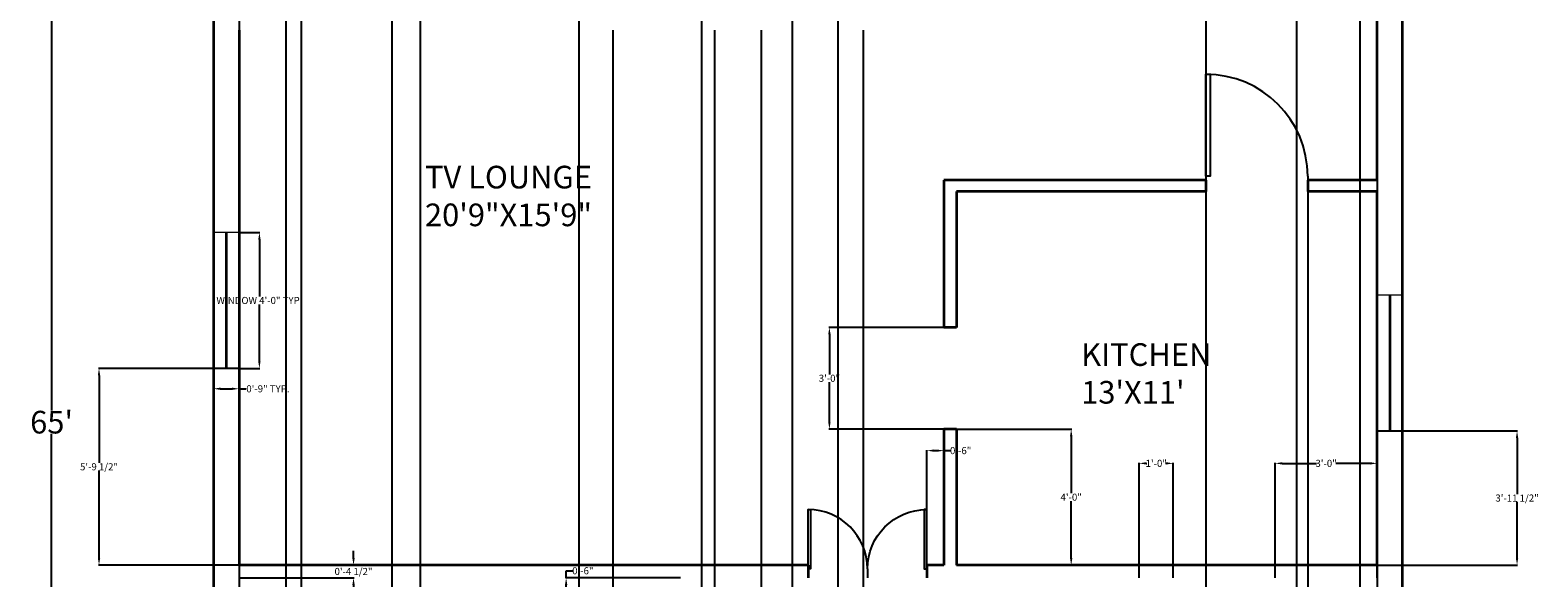
# Model space of a CAD drawing. Units: inches. Extents: x 1737 to 2270, y 2551 to 3419.
# Tile 3 of 4: x 1737 to 2270, y 2930 to 3124. Entities that reach past the tile are written whole.
import ezdxf

# ---------------------------------------------------------------- set-up
doc = ezdxf.new("R2010")
doc.units = ezdxf.units.IN
doc.header["$MEASUREMENT"] = 0
doc.layers.get('0').update_dxf_attribs({"color": 60})
for name, color, linetype, lineweight in [('A-ANNO-DIMS', 2, 'Continuous', 18), ('A-AREA-IDEN', 231, 'Continuous', 18), ('DOOR', 20, 'Continuous', 25), ('WALL', 60, 'Continuous', 35), ('WINDOW', 30, 'Continuous', 18)]:
    doc.layers.add(name, color=color, linetype=linetype, lineweight=lineweight)
doc.styles.get("Standard").update_dxf_attribs({"font": 'arial.ttf'})
doc.dimstyles.get("Standard").update_dxf_attribs({"dimtxt": 2.5, "dimasz": 2.5, "dimexe": 0.18, "dimexo": 0.0625, "dimgap": 0.09, "dimtad": 0, "dimtih": 1, "dimtoh": 1, "dimzin": 0, "dimdsep": 46, "dimlunit": 3, "dimtxsty": 'Standard', "dimcen": 0.09, "dimadec": 0, "dimazin": 0, "dimtfac": 1, "dimtofl": 0, "dimtmove": 0, "dimatfit": 3, "dimfxl": 1, "dimtolj": 1, "dimtzin": 0, "dimarcsym": 0})

# ---------------------------------------------------------------- blocks, each defined once
blk = doc.blocks.new('*U2')
for p, q in [((0, 0), (0, -6)), ((40, 0), (40, -6))]:
    blk.add_line(p, q)
blk.add_lwpolyline([(0, 0), (0, 40), (1.75, 40), (1.75, 0)], close=True)
blk.add_arc((0, 0), 40, 0, 90)
blk = doc.blocks.new('*D5')
at = {"layer": 'A-ANNO-DIMS', "color": 0, "lineweight": -2, "transparency": 16777216}
for p, q in [((1802.15, 3375.16), (1744.83, 3375.16)), ((1745.01, 3372.66), (1745.01, 2989.33)), ((1745.01, 2597.66), (1745.01, 2980.98)), ((1802.15, 2595.16), (1744.83, 2595.16))]:
    blk.add_line(p, q, dxfattribs=at)
at = {"layer": 'A-ANNO-DIMS', "color": 0, "transparency": 16777216}
for points in [[(1744.59, 3372.66), (1745.42, 3372.66), (1745.01, 3375.16)], [(1744.59, 2597.66), (1745.42, 2597.66), (1745.01, 2595.16)]]:
    blk.add_solid(points, dxfattribs=at)
at = {"layer": 'Defpoints', "color": 0, "transparency": 16777216}
for p in [(1802.21, 3375.16), (1745.01, 2595.16), (1802.21, 2595.16)]:
    blk.add_point(p, dxfattribs=at)
at = {"layer": 'A-ANNO-DIMS', "color": 0, "transparency": 16777216, "insert": (1745.01, 2985.16), "char_height": 8, "attachment_point": 5}
blk.add_mtext("\\A1;65'", dxfattribs=at)
blk = doc.blocks.new('WIN-48IN')
for p, q in [((4.25, 48), (4.25, 0)), ((4.75, 48), (4.75, 0))]:
    blk.add_line(p, q)
blk.add_lwpolyline([(0, 48), (0, 0), (9, 0), (9, 48)], close=True)
blk = doc.blocks.new('*D9')
at = {"layer": 'A-ANNO-DIMS', "color": 0, "lineweight": -2, "transparency": 16777216}
for p, q in [((1811.27, 3052.16), (1818.59, 3052.16)), ((1818.41, 3049.66), (1818.41, 3029.55)), ((1818.41, 3006.66), (1818.41, 3026.78)), ((1811.27, 3004.16), (1818.59, 3004.16))]:
    blk.add_line(p, q, dxfattribs=at)
at = {"layer": 'A-ANNO-DIMS', "color": 0, "transparency": 16777216}
for points in [[(1817.99, 3049.66), (1818.83, 3049.66), (1818.41, 3052.16)], [(1817.99, 3006.66), (1818.83, 3006.66), (1818.41, 3004.16)]]:
    blk.add_solid(points, dxfattribs=at)
at = {"layer": 'Defpoints', "color": 0, "transparency": 16777216}
for p in [(1811.21, 3052.16), (1818.41, 3052.16), (1811.21, 3004.16)]:
    blk.add_point(p, dxfattribs=at)
at = {"layer": 'A-ANNO-DIMS', "color": 0, "transparency": 16777216, "insert": (1818.41, 3028.16), "char_height": 2.5, "attachment_point": 5}
blk.add_mtext('\\A1;WINDOW 4\'-0" TYP.', dxfattribs=at)
blk = doc.blocks.new('*D10')
at = {"layer": 'A-ANNO-DIMS', "color": 0, "lineweight": -2, "transparency": 16777216}
for p, q in [((1802.21, 3004.1), (1802.21, 2996.78)), ((1811.21, 3004.1), (1811.21, 2996.78)), ((1804.71, 2996.96), (1808.71, 2996.96)), ((1811.21, 2996.96), (1813.71, 2996.96))]:
    blk.add_line(p, q, dxfattribs=at)
at = {"layer": 'A-ANNO-DIMS', "color": 0, "transparency": 16777216}
for points in [[(1804.71, 2997.38), (1804.71, 2996.55), (1802.21, 2996.96)], [(1808.71, 2997.38), (1808.71, 2996.55), (1811.21, 2996.96)]]:
    blk.add_solid(points, dxfattribs=at)
at = {"layer": 'Defpoints', "color": 0, "transparency": 16777216}
for p in [(1802.21, 3004.16), (1811.21, 3004.16), (1811.21, 2996.96)]:
    blk.add_point(p, dxfattribs=at)
at = {"layer": 'A-ANNO-DIMS', "color": 0, "transparency": 16777216, "insert": (1821.42, 2996.96), "char_height": 2.5, "attachment_point": 5}
blk.add_mtext('\\A1;0\'-9" TYP.', dxfattribs=at)
blk = doc.blocks.new('*D14')
at = {"layer": 'A-ANNO-DIMS', "color": 0, "lineweight": -2, "transparency": 16777216}
for p, q in [((1811.15, 3004.16), (1761.58, 3004.16)), ((1761.76, 3001.66), (1761.76, 2970.79)), ((1761.76, 2937.16), (1761.76, 2968.03)), ((1811.15, 2934.66), (1761.58, 2934.66))]:
    blk.add_line(p, q, dxfattribs=at)
at = {"layer": 'A-ANNO-DIMS', "color": 0, "transparency": 16777216}
for points in [[(1761.34, 3001.66), (1762.18, 3001.66), (1761.76, 3004.16)], [(1761.34, 2937.16), (1762.18, 2937.16), (1761.76, 2934.66)]]:
    blk.add_solid(points, dxfattribs=at)
at = {"layer": 'Defpoints', "color": 0, "transparency": 16777216}
for p in [(1761.76, 3004.16), (1811.21, 3004.16), (1811.21, 2934.66)]:
    blk.add_point(p, dxfattribs=at)
at = {"layer": 'A-ANNO-DIMS', "color": 0, "transparency": 16777216, "insert": (1761.76, 2969.41), "char_height": 2.5, "attachment_point": 5}
blk.add_mtext('\\A1;5\'-9 1/2"', dxfattribs=at)
blk = doc.blocks.new('*D16')
at = {"layer": 'A-ANNO-DIMS', "color": 0, "lineweight": -2, "transparency": 16777216}
for p, q in [((2213.27, 2982.05), (2262.84, 2982.05)), ((2262.66, 2979.55), (2262.66, 2959.74)), ((2262.66, 2937.16), (2262.66, 2956.97)), ((2213.27, 2934.66), (2262.84, 2934.66))]:
    blk.add_line(p, q, dxfattribs=at)
at = {"layer": 'A-ANNO-DIMS', "color": 0, "transparency": 16777216}
for points in [[(2262.24, 2979.55), (2263.08, 2979.55), (2262.66, 2982.05)], [(2262.24, 2937.16), (2263.08, 2937.16), (2262.66, 2934.66)]]:
    blk.add_solid(points, dxfattribs=at)
at = {"layer": 'Defpoints', "color": 0, "transparency": 16777216}
for p in [(2213.21, 2982.05), (2262.66, 2982.05), (2213.21, 2934.66)]:
    blk.add_point(p, dxfattribs=at)
at = {"layer": 'A-ANNO-DIMS', "color": 0, "transparency": 16777216, "insert": (2262.66, 2958.35), "char_height": 2.5, "attachment_point": 5}
blk.add_mtext('\\A1;3\'-11 1/2"', dxfattribs=at)
blk = doc.blocks.new('*D18')
at = {"layer": 'A-ANNO-DIMS', "color": 0, "lineweight": -2, "transparency": 16777216}
for p, q in [((1811.21, 3366.1), (1811.21, 2554.53)), ((1827.73, 3366.1), (1827.73, 2554.53)), ((1808.71, 2554.71), (1806.21, 2554.71)), ((1830.23, 2554.71), (1832.73, 2554.71))]:
    blk.add_line(p, q, dxfattribs=at)
at = {"layer": 'A-ANNO-DIMS', "color": 0, "transparency": 16777216}
for points in [[(1808.71, 2555.12), (1808.71, 2554.29), (1811.21, 2554.71)], [(1830.23, 2555.12), (1830.23, 2554.29), (1827.73, 2554.71)]]:
    blk.add_solid(points, dxfattribs=at)
at = {"layer": 'Defpoints', "color": 0, "transparency": 16777216}
for p in [(1811.21, 3366.16), (1827.73, 3366.16), (1827.73, 2554.71)]:
    blk.add_point(p, dxfattribs=at)
at = {"layer": 'A-ANNO-DIMS', "color": 0, "transparency": 16777216, "insert": (1819.47, 2554.71), "char_height": 2.5, "attachment_point": 5}
blk.add_mtext('\\A1;1\'-4 1/2"', dxfattribs=at)
blk = doc.blocks.new('*D20')
at = {"layer": 'A-ANNO-DIMS', "color": 0, "lineweight": -2, "transparency": 16777216}
for p, q in [((2022.87, 2595.22), (2022.87, 3415.79)), ((2025.37, 3415.61), (2107.86, 3415.61)), ((2204.71, 3415.61), (2122.22, 3415.61)), ((2207.21, 2595.22), (2207.21, 3415.79))]:
    blk.add_line(p, q, dxfattribs=at)
at = {"layer": 'A-ANNO-DIMS', "color": 0, "transparency": 16777216}
for points in [[(2025.37, 3416.02), (2025.37, 3415.19), (2022.87, 3415.61)], [(2204.71, 3416.02), (2204.71, 3415.19), (2207.21, 3415.61)]]:
    blk.add_solid(points, dxfattribs=at)
at = {"layer": 'Defpoints', "color": 0, "transparency": 16777216}
for p in [(2207.21, 3415.61), (2022.87, 2595.16), (2207.21, 2595.16)]:
    blk.add_point(p, dxfattribs=at)
at = {"layer": 'A-ANNO-DIMS', "color": 0, "transparency": 16777216, "insert": (2115.04, 3415.61), "char_height": 2.5, "attachment_point": 5}
blk.add_mtext('\\A1;15\'-4 1/2"', dxfattribs=at)
blk = doc.blocks.new('*D23')
at = {"layer": 'A-ANNO-DIMS', "color": 0, "lineweight": -2, "transparency": 16777216}
for p, q in [((1943.21, 3123.6), (1943.21, 2554.53)), ((1979.21, 3123.6), (1979.21, 2554.53)), ((1945.71, 2554.71), (1957.8, 2554.71)), ((1976.71, 2554.71), (1964.62, 2554.71))]:
    blk.add_line(p, q, dxfattribs=at)
at = {"layer": 'A-ANNO-DIMS', "color": 0, "transparency": 16777216}
for points in [[(1945.71, 2555.12), (1945.71, 2554.29), (1943.21, 2554.71)], [(1976.71, 2555.12), (1976.71, 2554.29), (1979.21, 2554.71)]]:
    blk.add_solid(points, dxfattribs=at)
at = {"layer": 'Defpoints', "color": 0, "transparency": 16777216}
for p in [(1943.21, 3123.66), (1979.21, 3123.66), (1979.21, 2554.71)]:
    blk.add_point(p, dxfattribs=at)
at = {"layer": 'A-ANNO-DIMS', "color": 0, "transparency": 16777216, "insert": (1961.21, 2554.71), "char_height": 2.5, "attachment_point": 5}
blk.add_mtext('\\A1;3\'-0"', dxfattribs=at)
blk = doc.blocks.new('*D24')
at = {"layer": 'A-ANNO-DIMS', "color": 0, "lineweight": -2, "transparency": 16777216}
for p, q in [((1833.21, 3284.1), (1833.21, 2554.53)), ((1865.21, 3284.1), (1865.21, 2554.53)), ((1835.71, 2554.71), (1845.77, 2554.71)), ((1862.71, 2554.71), (1852.64, 2554.71))]:
    blk.add_line(p, q, dxfattribs=at)
at = {"layer": 'A-ANNO-DIMS', "color": 0, "transparency": 16777216}
for points in [[(1835.71, 2555.12), (1835.71, 2554.29), (1833.21, 2554.71)], [(1862.71, 2555.12), (1862.71, 2554.29), (1865.21, 2554.71)]]:
    blk.add_solid(points, dxfattribs=at)
at = {"layer": 'Defpoints', "color": 0, "transparency": 16777216}
for p in [(1833.21, 3284.16), (1865.21, 3284.16), (1865.21, 2554.71)]:
    blk.add_point(p, dxfattribs=at)
at = {"layer": 'A-ANNO-DIMS', "color": 0, "transparency": 16777216, "insert": (1849.21, 2554.71), "char_height": 2.5, "attachment_point": 5}
blk.add_mtext('\\A1;2\'-8"', dxfattribs=at)
blk = doc.blocks.new('*D26')
at = {"layer": 'A-ANNO-DIMS', "color": 0, "lineweight": -2, "transparency": 16777216}
for p, q in [((2060.15, 3018.66), (2019.58, 3018.66)), ((2019.76, 3016.16), (2019.76, 3002.03)), ((2019.76, 2985.16), (2019.76, 2999.29)), ((2060.15, 2982.66), (2019.58, 2982.66))]:
    blk.add_line(p, q, dxfattribs=at)
at = {"layer": 'A-ANNO-DIMS', "color": 0, "transparency": 16777216}
for points in [[(2019.34, 3016.16), (2020.18, 3016.16), (2019.76, 3018.66)], [(2019.34, 2985.16), (2020.18, 2985.16), (2019.76, 2982.66)]]:
    blk.add_solid(points, dxfattribs=at)
at = {"layer": 'Defpoints', "color": 0, "transparency": 16777216}
for p in [(2019.76, 3018.66), (2060.21, 3018.66), (2060.21, 2982.66)]:
    blk.add_point(p, dxfattribs=at)
at = {"layer": 'A-ANNO-DIMS', "color": 0, "transparency": 16777216, "insert": (2019.76, 3000.66), "char_height": 2.5, "attachment_point": 5}
blk.add_mtext('\\A1;3\'-0"', dxfattribs=at)
blk = doc.blocks.new('*D29')
at = {"layer": 'A-ANNO-DIMS', "color": 0, "lineweight": -2, "transparency": 16777216}
for p, q in [((1974.71, 2758.72), (1974.71, 3415.79)), ((1977.21, 3415.61), (1987.27, 3415.61)), ((2004.21, 3415.61), (1994.14, 3415.61)), ((2006.71, 2758.72), (2006.71, 3415.79))]:
    blk.add_line(p, q, dxfattribs=at)
at = {"layer": 'A-ANNO-DIMS', "color": 0, "transparency": 16777216}
for points in [[(1977.21, 3416.02), (1977.21, 3415.19), (1974.71, 3415.61)], [(2004.21, 3416.02), (2004.21, 3415.19), (2006.71, 3415.61)]]:
    blk.add_solid(points, dxfattribs=at)
at = {"layer": 'Defpoints', "color": 0, "transparency": 16777216}
for p in [(2006.71, 3415.61), (1974.71, 2758.66), (2006.71, 2758.66)]:
    blk.add_point(p, dxfattribs=at)
at = {"layer": 'A-ANNO-DIMS', "color": 0, "transparency": 16777216, "insert": (1990.71, 3415.61), "char_height": 2.5, "attachment_point": 5}
blk.add_mtext('\\A1;2\'-8"', dxfattribs=at)
blk = doc.blocks.new('*D31')
at = {"layer": 'A-ANNO-DIMS', "color": 0, "lineweight": -2, "transparency": 16777216}
for p, q in [((2129.21, 2930.22), (2129.21, 2970.79)), ((2131.71, 2970.61), (2131.91, 2970.61)), ((2138.71, 2970.61), (2138.5, 2970.61)), ((2141.21, 2930.22), (2141.21, 2970.79))]:
    blk.add_line(p, q, dxfattribs=at)
at = {"layer": 'A-ANNO-DIMS', "color": 0, "transparency": 16777216}
for points in [[(2131.71, 2971.02), (2131.71, 2970.19), (2129.21, 2970.61)], [(2138.71, 2971.02), (2138.71, 2970.19), (2141.21, 2970.61)]]:
    blk.add_solid(points, dxfattribs=at)
at = {"layer": 'Defpoints', "color": 0, "transparency": 16777216}
for p in [(2141.21, 2970.61), (2129.21, 2930.16), (2141.21, 2930.16)]:
    blk.add_point(p, dxfattribs=at)
at = {"layer": 'A-ANNO-DIMS', "color": 0, "transparency": 16777216, "insert": (2135.21, 2970.61), "char_height": 2.5, "attachment_point": 5}
blk.add_mtext('\\A1;1\'-0"', dxfattribs=at)
blk = doc.blocks.new('*D32')
at = {"layer": 'A-ANNO-DIMS', "color": 0, "lineweight": -2, "transparency": 16777216}
for p, q in [((2177.21, 2930.22), (2177.21, 2970.79)), ((2179.71, 2970.61), (2191.8, 2970.61)), ((2210.71, 2970.61), (2198.62, 2970.61)), ((2213.21, 2930.22), (2213.21, 2970.79))]:
    blk.add_line(p, q, dxfattribs=at)
at = {"layer": 'A-ANNO-DIMS', "color": 0, "transparency": 16777216}
for points in [[(2179.71, 2971.02), (2179.71, 2970.19), (2177.21, 2970.61)], [(2210.71, 2971.02), (2210.71, 2970.19), (2213.21, 2970.61)]]:
    blk.add_solid(points, dxfattribs=at)
at = {"layer": 'Defpoints', "color": 0, "transparency": 16777216}
for p in [(2213.21, 2970.61), (2177.21, 2930.16), (2213.21, 2930.16)]:
    blk.add_point(p, dxfattribs=at)
at = {"layer": 'A-ANNO-DIMS', "color": 0, "transparency": 16777216, "insert": (2195.21, 2970.61), "char_height": 2.5, "attachment_point": 5}
blk.add_mtext('\\A1;3\'-0"', dxfattribs=at)
blk = doc.blocks.new('*D34')
at = {"layer": 'A-ANNO-DIMS', "color": 0, "lineweight": -2, "transparency": 16777216}
for p, q in [((1995.71, 3123.6), (1995.71, 2554.53)), ((2031.71, 3123.6), (2031.71, 2554.53)), ((1998.21, 2554.71), (2010.3, 2554.71)), ((2029.21, 2554.71), (2017.12, 2554.71))]:
    blk.add_line(p, q, dxfattribs=at)
at = {"layer": 'A-ANNO-DIMS', "color": 0, "transparency": 16777216}
for points in [[(1998.21, 2555.12), (1998.21, 2554.29), (1995.71, 2554.71)], [(2029.21, 2555.12), (2029.21, 2554.29), (2031.71, 2554.71)]]:
    blk.add_solid(points, dxfattribs=at)
at = {"layer": 'Defpoints', "color": 0, "transparency": 16777216}
for p in [(1995.71, 3123.66), (2031.71, 3123.66), (2031.71, 2554.71)]:
    blk.add_point(p, dxfattribs=at)
at = {"layer": 'A-ANNO-DIMS', "color": 0, "transparency": 16777216, "insert": (2013.71, 2554.71), "char_height": 2.5, "attachment_point": 5}
blk.add_mtext('\\A1;3\'-0"', dxfattribs=at)
blk = doc.blocks.new('*D35')
at = {"layer": 'A-ANNO-DIMS', "color": 0, "lineweight": -2, "transparency": 16777216}
for p, q in [((2152.71, 3066.6), (2152.71, 2554.53)), ((2188.71, 3066.6), (2188.71, 2554.53)), ((2155.21, 2554.71), (2167.3, 2554.71)), ((2186.21, 2554.71), (2174.12, 2554.71))]:
    blk.add_line(p, q, dxfattribs=at)
at = {"layer": 'A-ANNO-DIMS', "color": 0, "transparency": 16777216}
for points in [[(2155.21, 2555.12), (2155.21, 2554.29), (2152.71, 2554.71)], [(2186.21, 2555.12), (2186.21, 2554.29), (2188.71, 2554.71)]]:
    blk.add_solid(points, dxfattribs=at)
at = {"layer": 'Defpoints', "color": 0, "transparency": 16777216}
for p in [(2152.71, 3066.66), (2188.71, 3066.66), (2188.71, 2554.71)]:
    blk.add_point(p, dxfattribs=at)
at = {"layer": 'A-ANNO-DIMS', "color": 0, "transparency": 16777216, "insert": (2170.71, 2554.71), "char_height": 2.5, "attachment_point": 5}
blk.add_mtext('\\A1;3\'-0"', dxfattribs=at)
blk = doc.blocks.new('*D36')
at = {"layer": 'A-ANNO-DIMS', "color": 0, "lineweight": -2, "transparency": 16777216}
for p, q in [((2152.71, 3260.1), (2152.71, 2554.53)), ((2184.71, 3260.1), (2184.71, 2554.53)), ((2155.21, 2554.71), (2165.27, 2554.71)), ((2182.21, 2554.71), (2172.14, 2554.71))]:
    blk.add_line(p, q, dxfattribs=at)
at = {"layer": 'A-ANNO-DIMS', "color": 0, "transparency": 16777216}
for points in [[(2155.21, 2555.12), (2155.21, 2554.29), (2152.71, 2554.71)], [(2182.21, 2555.12), (2182.21, 2554.29), (2184.71, 2554.71)]]:
    blk.add_solid(points, dxfattribs=at)
at = {"layer": 'Defpoints', "color": 0, "transparency": 16777216}
for p in [(2152.71, 3260.16), (2184.71, 3260.16), (2184.71, 2554.71)]:
    blk.add_point(p, dxfattribs=at)
at = {"layer": 'A-ANNO-DIMS', "color": 0, "transparency": 16777216, "insert": (2168.71, 2554.71), "char_height": 2.5, "attachment_point": 5}
blk.add_mtext('\\A1;2\'-8"', dxfattribs=at)
blk = doc.blocks.new('*D37')
at = {"layer": 'A-ANNO-DIMS', "color": 0, "lineweight": -2, "transparency": 16777216}
for p, q in [((2064.77, 2982.66), (2105.34, 2982.66)), ((2105.16, 2980.16), (2105.16, 2960.02)), ((2105.16, 2937.16), (2105.16, 2957.29)), ((2064.77, 2934.66), (2105.34, 2934.66))]:
    blk.add_line(p, q, dxfattribs=at)
at = {"layer": 'A-ANNO-DIMS', "color": 0, "transparency": 16777216}
for points in [[(2104.74, 2980.16), (2105.58, 2980.16), (2105.16, 2982.66)], [(2104.74, 2937.16), (2105.58, 2937.16), (2105.16, 2934.66)]]:
    blk.add_solid(points, dxfattribs=at)
at = {"layer": 'Defpoints', "color": 0, "transparency": 16777216}
for p in [(2064.71, 2982.66), (2064.71, 2934.66), (2105.16, 2934.66)]:
    blk.add_point(p, dxfattribs=at)
at = {"layer": 'A-ANNO-DIMS', "color": 0, "transparency": 16777216, "insert": (2105.16, 2958.66), "char_height": 2.5, "attachment_point": 5}
blk.add_mtext('\\A1;4\'-0"', dxfattribs=at)
blk = doc.blocks.new('*D39')
at = {"layer": 'A-ANNO-DIMS', "color": 0, "lineweight": -2, "transparency": 16777216}
for p, q in [((1875.21, 3366.1), (1875.21, 2554.53)), ((1931.21, 3366.1), (1931.21, 2554.53)), ((1877.71, 2554.71), (1899.75, 2554.71)), ((1928.71, 2554.71), (1906.67, 2554.71))]:
    blk.add_line(p, q, dxfattribs=at)
at = {"layer": 'A-ANNO-DIMS', "color": 0, "transparency": 16777216}
for points in [[(1877.71, 2555.12), (1877.71, 2554.29), (1875.21, 2554.71)], [(1928.71, 2555.12), (1928.71, 2554.29), (1931.21, 2554.71)]]:
    blk.add_solid(points, dxfattribs=at)
at = {"layer": 'Defpoints', "color": 0, "transparency": 16777216}
for p in [(1875.21, 3366.16), (1931.21, 3366.16), (1931.21, 2554.71)]:
    blk.add_point(p, dxfattribs=at)
at = {"layer": 'A-ANNO-DIMS', "color": 0, "transparency": 16777216, "insert": (1903.21, 2554.71), "char_height": 2.5, "attachment_point": 5}
blk.add_mtext('\\A1;4\'-8"', dxfattribs=at)
blk = doc.blocks.new('*D42')
at = {"layer": 'A-ANNO-DIMS', "color": 0, "lineweight": -2, "transparency": 16777216}
for p, q in [((2184.71, 3263.5), (2184.71, 2554.53)), ((2213.21, 3264.1), (2213.21, 2554.53)), ((2187.21, 2554.71), (2192.61, 2554.71)), ((2210.71, 2554.71), (2205.31, 2554.71))]:
    blk.add_line(p, q, dxfattribs=at)
at = {"layer": 'A-ANNO-DIMS', "color": 0, "transparency": 16777216}
for points in [[(2187.21, 2555.12), (2187.21, 2554.29), (2184.71, 2554.71)], [(2210.71, 2555.12), (2210.71, 2554.29), (2213.21, 2554.71)]]:
    blk.add_solid(points, dxfattribs=at)
at = {"layer": 'Defpoints', "color": 0, "transparency": 16777216}
for p in [(2184.71, 3263.56), (2213.21, 3264.16), (2213.21, 2554.71)]:
    blk.add_point(p, dxfattribs=at)
at = {"layer": 'A-ANNO-DIMS', "color": 0, "transparency": 16777216, "insert": (2198.96, 2554.71), "char_height": 2.5, "attachment_point": 5}
blk.add_mtext('\\A1;2\'-4 1/2"', dxfattribs=at)
blk = doc.blocks.new('*D43')
at = {"layer": 'A-ANNO-DIMS', "color": 0, "lineweight": -2, "transparency": 16777216}
for p, q in [((2188.71, 3066.6), (2188.71, 2554.53)), ((2213.21, 3066.6), (2213.21, 2554.53)), ((2191.21, 2554.71), (2194.61, 2554.71)), ((2210.71, 2554.71), (2207.31, 2554.71))]:
    blk.add_line(p, q, dxfattribs=at)
at = {"layer": 'A-ANNO-DIMS', "color": 0, "transparency": 16777216}
for points in [[(2191.21, 2555.12), (2191.21, 2554.29), (2188.71, 2554.71)], [(2210.71, 2555.12), (2210.71, 2554.29), (2213.21, 2554.71)]]:
    blk.add_solid(points, dxfattribs=at)
at = {"layer": 'Defpoints', "color": 0, "transparency": 16777216}
for p in [(2188.71, 3066.66), (2213.21, 3066.66), (2213.21, 2554.71)]:
    blk.add_point(p, dxfattribs=at)
at = {"layer": 'A-ANNO-DIMS', "color": 0, "transparency": 16777216, "insert": (2200.96, 2554.71), "char_height": 2.5, "attachment_point": 5}
blk.add_mtext('\\A1;2\'-0 1/2"', dxfattribs=at)
blk = doc.blocks.new('*D47')
at = {"layer": 'A-ANNO-DIMS', "color": 0, "lineweight": -2, "transparency": 16777216}
for p, q in [((1967.15, 2930.16), (1926.58, 2930.16)), ((1926.76, 2930.16), (1926.76, 2932.66)), ((1926.76, 2932.66), (1929.26, 2932.66)), ((1967.15, 2924.16), (1926.58, 2924.16)), ((1926.76, 2926.66), (1926.76, 2927.66))]:
    blk.add_line(p, q, dxfattribs=at)
at = {"layer": 'A-ANNO-DIMS', "color": 0, "transparency": 16777216}
for points in [[(1926.34, 2927.66), (1927.18, 2927.66), (1926.76, 2930.16)], [(1926.34, 2926.66), (1927.18, 2926.66), (1926.76, 2924.16)]]:
    blk.add_solid(points, dxfattribs=at)
at = {"layer": 'Defpoints', "color": 0, "transparency": 16777216}
for p in [(1926.76, 2930.16), (1967.21, 2930.16), (1967.21, 2924.16)]:
    blk.add_point(p, dxfattribs=at)
at = {"layer": 'A-ANNO-DIMS', "color": 0, "transparency": 16777216, "insert": (1932.67, 2932.66), "char_height": 2.5, "attachment_point": 5}
blk.add_mtext('\\A1;0\'-6"', dxfattribs=at)
blk = doc.blocks.new('*D48')
at = {"layer": 'A-ANNO-DIMS', "color": 0, "lineweight": -2, "transparency": 16777216}
for p, q in [((2054.21, 2934.72), (2054.21, 2975.29)), ((2056.71, 2975.11), (2057.71, 2975.11)), ((2060.21, 2934.72), (2060.21, 2975.29)), ((2060.21, 2975.11), (2062.71, 2975.11))]:
    blk.add_line(p, q, dxfattribs=at)
at = {"layer": 'A-ANNO-DIMS', "color": 0, "transparency": 16777216}
for points in [[(2056.71, 2975.52), (2056.71, 2974.69), (2054.21, 2975.11)], [(2057.71, 2975.52), (2057.71, 2974.69), (2060.21, 2975.11)]]:
    blk.add_solid(points, dxfattribs=at)
at = {"layer": 'Defpoints', "color": 0, "transparency": 16777216}
for p in [(2060.21, 2975.11), (2054.21, 2934.66), (2060.21, 2934.66)]:
    blk.add_point(p, dxfattribs=at)
at = {"layer": 'A-ANNO-DIMS', "color": 0, "transparency": 16777216, "insert": (2066.12, 2975.11), "char_height": 2.5, "attachment_point": 5}
blk.add_mtext('\\A1;0\'-6"', dxfattribs=at)
blk = doc.blocks.new('*D51')
at = {"layer": 'A-ANNO-DIMS', "color": 0, "lineweight": -2, "transparency": 16777216}
for p, q in [((1811.27, 2934.66), (1851.84, 2934.66)), ((1851.66, 2937.16), (1851.66, 2939.66)), ((1811.27, 2930.16), (1851.84, 2930.16)), ((1851.66, 2927.66), (1851.66, 2925.16))]:
    blk.add_line(p, q, dxfattribs=at)
at = {"layer": 'A-ANNO-DIMS', "color": 0, "transparency": 16777216}
for points in [[(1851.24, 2937.16), (1852.08, 2937.16), (1851.66, 2934.66)], [(1851.24, 2927.66), (1852.08, 2927.66), (1851.66, 2930.16)]]:
    blk.add_solid(points, dxfattribs=at)
at = {"layer": 'Defpoints', "color": 0, "transparency": 16777216}
for p in [(1811.21, 2934.66), (1811.21, 2930.16), (1851.66, 2930.16)]:
    blk.add_point(p, dxfattribs=at)
at = {"layer": 'A-ANNO-DIMS', "color": 0, "transparency": 16777216, "insert": (1851.66, 2932.41), "char_height": 2.5, "attachment_point": 5}
blk.add_mtext('\\A1;0\'-4 1/2"', dxfattribs=at)

msp = doc.modelspace()

# ---------------------------------------------------------------- linework, layer by layer
at = {"layer": 'WALL'}
for p, q in [((1802.209, 3375.158), (1802.209, 2669.158)), ((2222.209, 2595.158), (2222.209, 3375.158)), ((2213.209, 3070.658), (2213.209, 3190.158)), ((1811.209, 3123.658), (1811.209, 2934.658)), ((2060.209, 3070.658), (2060.209, 3018.658)), ((2152.709, 3070.658), (2060.209, 3070.658)), ((2152.709, 3070.658), (2152.709, 3066.658)), ((2213.209, 3070.658), (2188.709, 3070.658)), ((2188.709, 3070.658), (2188.709, 3066.658)), ((2064.709, 3066.658), (2064.709, 3018.658)), ((2152.709, 3066.658), (2064.709, 3066.658)), ((2213.209, 3066.658), (2188.709, 3066.658)), ((2213.209, 2934.658), (2213.209, 3066.658)), ((2064.709, 3018.658), (2060.209, 3018.658)), ((2064.709, 2982.658), (2060.209, 2982.658)), ((2060.209, 2982.658), (2060.209, 2934.658)), ((2064.709, 2982.658), (2064.709, 2934.658)), ((2012.209, 2934.658), (1811.209, 2934.658)), ((2012.209, 2934.658), (2012.209, 2930.158)), ((2060.209, 2934.658), (2054.209, 2934.658)), ((2054.209, 2934.658), (2054.209, 2930.158)), ((2213.209, 2934.658), (2064.709, 2934.658))]:
    msp.add_line(p, q, dxfattribs=at)

# ---------------------------------------------------------------- block references
at = {"layer": 'DOOR'}
for p, xscale, yscale, zscale in [((2152.709, 3072.058), 0.8999999999999948, 0.8999999999999948, 0.8999999999999948), ((2012.209, 2933.308), 0.5249999999999972, 0.5249999999999972, 0.5249999999999972), ((2054.209, 2933.308), -0.5249999999999972, 0.5249999999999972, 0.5249999999999972)]:
    msp.add_blockref('*U2', p, dxfattribs=dict(at, xscale=xscale, yscale=yscale, zscale=zscale))
at = {"layer": 'WINDOW'}
for p in [(1802.209, 3004.164), (2213.209, 2982.048)]:
    msp.add_blockref('WIN-48IN', p, dxfattribs=at)

# ---------------------------------------------------------------- texts
at = {"layer": 'A-AREA-IDEN', "char_height": 8, "attachment_point": 1}
for s, width, insert in [('TV LOUNGE\\P20\'9"X15\'9"', 70.55036, (1876.891, 3075.736)), ("KITCHEN\\P13'X11'", 60.91246, (2108.681, 3013.041))]:
    msp.add_mtext_dynamic_manual_height_columns(s, width=width, gutter_width=1, heights=[0], dxfattribs=dict(at, insert=insert))

# ---------------------------------------------------------------- dimensions: what is measured, and where the dimension line sits
at = {"layer": 'A-ANNO-DIMS'}
for base, p1, p2, picture, middle in [((2207.209, 3415.608), (2022.872, 2595.158), (2207.209, 2595.158), '*D20', (2115.041, 3415.608)), ((2006.709, 3415.608), (1974.709, 2758.658), (2006.709, 2758.658), '*D29', (1990.709, 3415.608)), ((1827.725, 2554.708), (1811.209, 3366.158), (1827.725, 3366.158), '*D18', (1819.467, 2554.708)), ((1931.209, 2554.708), (1875.209, 3366.158), (1931.209, 3366.158), '*D39', (1903.209, 2554.708)), ((1865.209, 2554.708), (1833.209, 3284.158), (1865.209, 3284.158), '*D24', (1849.209, 2554.708)), ((2184.709, 2554.708), (2152.709, 3260.158), (2184.709, 3260.158), '*D36', (2168.709, 2554.708)), ((2213.209, 2554.708), (2184.709, 3263.558), (2213.209, 3264.158), '*D42', (2198.959, 2554.708)), ((1979.209, 2554.708), (1943.209, 3123.658), (1979.209, 3123.658), '*D23', (1961.209, 2554.708)), ((2031.709, 2554.708), (1995.709, 3123.658), (2031.709, 3123.658), '*D34', (2013.709, 2554.708)), ((2188.709, 2554.708), (2152.709, 3066.658), (2188.709, 3066.658), '*D35', (2170.709, 2554.708)), ((2213.209, 2554.708), (2188.709, 3066.658), (2213.209, 3066.658), '*D43', (2200.959, 2554.708)), ((2060.209, 2975.108), (2054.209, 2934.658), (2060.209, 2934.658), '*D48', (2066.122, 2975.108)), ((2141.209, 2970.608), (2129.209, 2930.158), (2141.209, 2930.158), '*D31', (2135.209, 2970.608)), ((2213.209, 2970.608), (2177.209, 2930.158), (2213.209, 2930.158), '*D32', (2195.209, 2970.608))]:
    dim = msp.add_linear_dim(base=base, p1=p1, p2=p2, dimstyle='Standard', override={"dimdec": 1, "dimlfac": 1, "dimrnd": 0, "dimzin": 1, "dimdsep": 46, "dimlunit": 4, "dimfrac": 2}, dxfattribs=at)
    dim.commit()
    dim.dimension.update_dxf_attribs({"geometry": picture, "text_midpoint": middle})
dim = msp.add_aligned_dim(p1=(1802.209, 3375.158), p2=(1802.209, 2595.158), distance=-57.201, dimstyle='Standard', override={"dimtxt": 8, "dimclrd": 0, "dimclre": 0, "dimclrt": 0}, dxfattribs=at)
dim.commit()
dim.dimension.update_dxf_attribs({"geometry": '*D5', "text_midpoint": (1745.008, 2985.158)})
dim = msp.add_linear_dim(base=(1818.409, 3052.164), p1=(1811.209, 3004.164), p2=(1811.209, 3052.164), angle=90, text='WINDOW <> TYP.', dimstyle='Standard', override={"dimdec": 1, "dimlfac": 1, "dimrnd": 0, "dimzin": 1, "dimdsep": 46, "dimlunit": 4, "dimfrac": 2}, dxfattribs=at)
dim.commit()
dim.dimension.update_dxf_attribs({"geometry": '*D9', "text_midpoint": (1818.409, 3028.164)})
for base, p1, p2, angle, picture, middle in [((2019.759, 3018.658), (2060.209, 2982.658), (2060.209, 3018.658), 90, '*D26', (2019.759, 3000.658)), ((1761.759, 3004.164), (1811.209, 2934.658), (1811.209, 3004.164), 90, '*D14', (1761.759, 2969.411)), ((2105.159, 2934.658), (2064.709, 2982.658), (2064.709, 2934.658), 270, '*D37', (2105.159, 2958.658)), ((2262.659, 2982.048), (2213.209, 2934.658), (2213.209, 2982.048), 90, '*D16', (2262.659, 2958.353)), ((1851.659, 2930.158), (1811.209, 2934.658), (1811.209, 2930.158), 270, '*D51', (1851.659, 2932.408)), ((1926.759, 2930.158), (1967.209, 2924.158), (1967.209, 2930.158), 90, '*D47', (1932.672, 2932.658))]:
    dim = msp.add_linear_dim(base=base, p1=p1, p2=p2, angle=angle, dimstyle='Standard', override={"dimdec": 1, "dimlfac": 1, "dimrnd": 0, "dimzin": 1, "dimdsep": 46, "dimlunit": 4, "dimfrac": 2}, dxfattribs=at)
    dim.commit()
    dim.dimension.update_dxf_attribs({"geometry": picture, "text_midpoint": middle})
dim = msp.add_linear_dim(base=(1811.209, 2996.964), p1=(1802.209, 3004.164), p2=(1811.209, 3004.164), text='<> TYP.', dimstyle='Standard', override={"dimdec": 1, "dimlfac": 1, "dimrnd": 0, "dimzin": 1, "dimdsep": 46, "dimlunit": 4, "dimfrac": 2}, dxfattribs=at)
dim.commit()
dim.dimension.update_dxf_attribs({"geometry": '*D10', "text_midpoint": (1821.418, 2996.964)})

doc.saveas('drawing.dxf')
